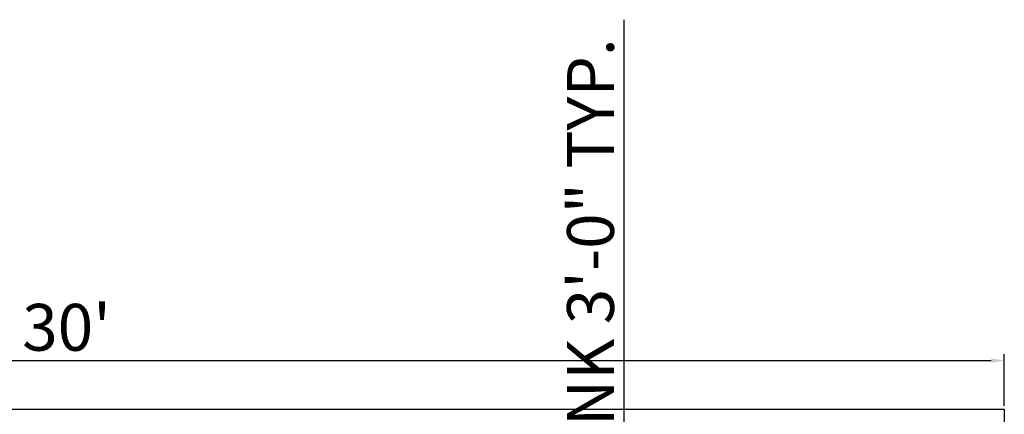
# Model space of a CAD drawing. Units: inches. Extents: x 2831 to 4250, y 1103 to 1797.
# Tile 13 of 15: x 3614 to 3803, y 1722 to 1797. Entities that reach past the tile are written whole.
import ezdxf

# ---------------------------------------------------------------- set-up
doc = ezdxf.new("R2010")
doc.units = ezdxf.units.IN
doc.layers.add('A-ANNO-DIMS', color=2, linetype='Continuous', lineweight=18)
doc.layers.add('C-PROP', color=7, linetype='Continuous', lineweight=25)
doc.styles.get("Standard").update_dxf_attribs({"font": 'arial.ttf'})
doc.dimstyles.new('ISO-25', dxfattribs={"dimtxt": 9, "dimasz": 2.5, "dimexe": 1.25, "dimexo": 0.625, "dimtad": 1, "dimdec": 1, "dimlunit": 3, "dimtxsty": 'Standard', "dimcen": 2.5, "dimadec": 0, "dimazin": 0, "dimtfac": 1, "dimtdec": 1, "dimtmove": 0, "dimatfit": 3, "dimfxl": 1, "dimarcsym": 0})

# ---------------------------------------------------------------- blocks, each defined once
blk = doc.blocks.new('*D5')
at = {"layer": 'A-ANNO-DIMS', "color": 0, "lineweight": -2, "transparency": 16777216}
for p, q in [((3443.23, 1723.14), (3443.23, 1733.1)), ((3445.73, 1731.85), (3800.73, 1731.85)), ((3803.23, 1723.14), (3803.23, 1733.1))]:
    blk.add_line(p, q, dxfattribs=at)
at = {"layer": 'A-ANNO-DIMS', "color": 0, "transparency": 16777216}
for points in [[(3445.73, 1732.27), (3445.73, 1731.43), (3443.23, 1731.85)], [(3800.73, 1732.27), (3800.73, 1731.43), (3803.23, 1731.85)]]:
    blk.add_solid(points, dxfattribs=at)
at = {"layer": 'Defpoints', "color": 0, "transparency": 16777216}
for p in [(3803.23, 1731.85), (3443.23, 1722.51), (3803.23, 1722.51)]:
    blk.add_point(p, dxfattribs=at)
at = {"layer": 'A-ANNO-DIMS', "color": 0, "transparency": 16777216, "insert": (3623.23, 1737.07), "char_height": 9, "attachment_point": 5}
blk.add_mtext("30'", dxfattribs=at)
blk = doc.blocks.new('*D85')
at = {"layer": 'A-ANNO-DIMS', "color": 0, "lineweight": -2, "transparency": 16777216}
for p, q in [((3730.24, 1651.15), (3730.24, 1797.34)), ((3735.01, 1651.15), (3728.99, 1651.15)), ((3730.24, 1617.65), (3730.24, 1648.65)), ((3735.01, 1615.15), (3728.99, 1615.15))]:
    blk.add_line(p, q, dxfattribs=at)
at = {"layer": 'A-ANNO-DIMS', "color": 0, "transparency": 16777216}
for points in [[(3729.82, 1648.65), (3730.66, 1648.65), (3730.24, 1651.15)], [(3729.82, 1617.65), (3730.66, 1617.65), (3730.24, 1615.15)]]:
    blk.add_solid(points, dxfattribs=at)
at = {"layer": 'Defpoints', "color": 0, "transparency": 16777216}
for p in [(3730.24, 1651.15), (3735.64, 1651.15), (3735.64, 1615.15)]:
    blk.add_point(p, dxfattribs=at)
at = {"layer": 'A-ANNO-DIMS', "color": 0, "transparency": 16777216, "insert": (3724.96, 1725.49), "char_height": 9, "attachment_point": 5, "rotation": 90}
blk.add_mtext('DOUBLE SINK 3\'-0" TYP.', dxfattribs=at)

msp = doc.modelspace()

# ---------------------------------------------------------------- linework, layer by layer
at = {"layer": 'C-PROP'}
msp.add_lwpolyline([(3443.23, 1722.51), (3803.23, 1722.51), (3803.23, 1242.51), (3443.23, 1242.51)], close=True, dxfattribs=at)

# ---------------------------------------------------------------- dimensions: what is measured, and where the dimension line sits
at = {"layer": 'A-ANNO-DIMS'}
dim = msp.add_linear_dim(base=(3730.24, 1651.15), p1=(3735.64, 1615.15), p2=(3735.64, 1651.15), angle=90, text='DOUBLE SINK <> TYP.', dimstyle='ISO-25', override={"dimdec": 1, "dimlfac": 1, "dimrnd": 0, "dimzin": 1, "dimdsep": 46, "dimlunit": 4, "dimfrac": 2}, dxfattribs=at)
dim.commit()
dim.dimension.update_dxf_attribs({"geometry": '*D85', "text_midpoint": (3724.96, 1725.49)})
dim = msp.add_linear_dim(base=(3803.23, 1731.85), p1=(3443.23, 1722.51), p2=(3803.23, 1722.51), dimstyle='ISO-25', override={"dimclrd": 0, "dimclre": 0, "dimclrt": 0}, dxfattribs=at)
dim.commit()
dim.dimension.update_dxf_attribs({"geometry": '*D5', "text_midpoint": (3623.23, 1737.07)})

doc.saveas('drawing.dxf')
